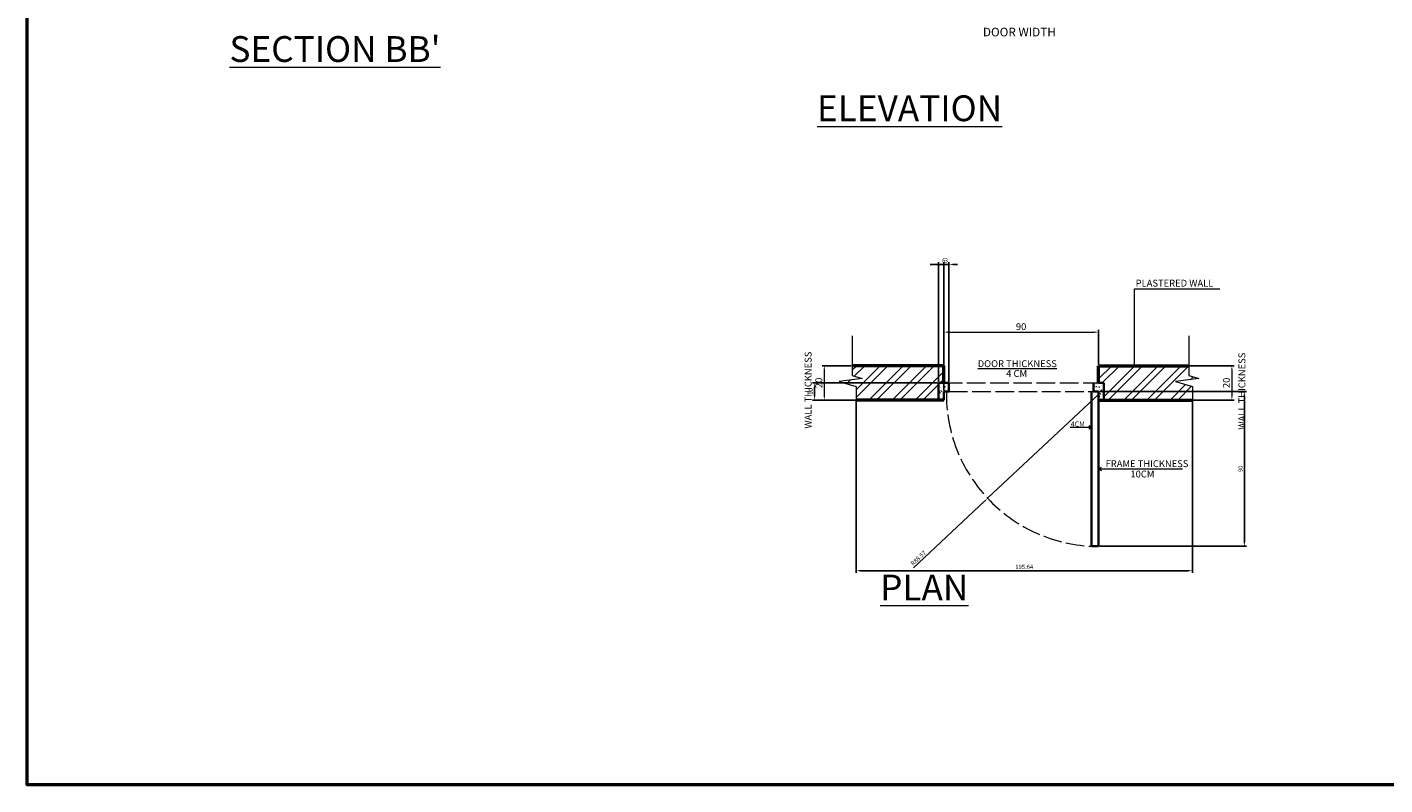
# Model space of a CAD drawing. Units: centimetres. Extents: x 1523 to 2760, y 1250 to 2134.
# Tile 1 of 4: x 1523 to 2313, y 1250 to 1691. Entities that reach past the tile are written whole.
import ezdxf

# ---------------------------------------------------------------- set-up
doc = ezdxf.new("R2010")
doc.units = ezdxf.units.CM
doc.linetypes.add('ACAD_ISO02W100', pattern=[15, 12, -3])
for name, color, linetype, lineweight in [('A-ANNO-DIMS', 2, 'Continuous', 18), ('A-ANNO-SYMB', 7, 'Continuous', 18), ('A-ANNO-TEXT', 7, 'Continuous', 18), ('A-ANNO-TTLB', 7, 'Continuous', 50), ('A-DOOR', 4, 'Continuous', 35), ('A-DOOR-OVHD', 252, 'ACAD_ISO02W100', 18), ('A-DOOR-PATT', 251, 'Continuous', 13), ('A-WALL', 7, 'Continuous', 50), ('A-WALL-PATT', 251, 'Continuous', 13)]:
    doc.layers.add(name, color=color, linetype=linetype, lineweight=lineweight)
doc.styles.get("Standard").update_dxf_attribs({"font": 'arial.ttf'})
doc.dimstyles.new('ISO-25', dxfattribs={"dimtxt": 2.5, "dimasz": 2.5, "dimexe": 1.25, "dimexo": 0.625, "dimtad": 1, "dimtxsty": 'Standard', "dimcen": 2.5, "dimadec": 0, "dimazin": 0, "dimtfac": 1, "dimtmove": 0, "dimatfit": 3, "dimfxl": 1, "dimarcsym": 0})

# ---------------------------------------------------------------- blocks, each defined once
blk = doc.blocks.new('*D1')
at = {"layer": 'A-ANNO-DIMS', "color": 0, "lineweight": -2, "transparency": 16777216}
for p, q in [((2056.32, 1494.6), (2056.32, 1514.72)), ((2146.32, 1494.6), (2146.32, 1514.72))]:
    blk.add_line(p, q, dxfattribs=at)
at = {"layer": 'A-ANNO-DIMS', "color": 0, "lineweight": 0, "transparency": 16777216}
blk.add_line((2058.82, 1513.47), (2143.82, 1513.47), dxfattribs=at)
at = {"layer": 'A-ANNO-DIMS', "color": 0, "transparency": 16777216}
for points in [[(2058.82, 1513.89), (2058.82, 1513.06), (2056.32, 1513.47)], [(2143.82, 1513.89), (2143.82, 1513.06), (2146.32, 1513.47)]]:
    blk.add_solid(points, dxfattribs=at)
at = {"layer": 'Defpoints', "color": 0, "transparency": 16777216}
for p in [(2146.32, 1513.47), (2056.32, 1493.97), (2146.32, 1493.97)]:
    blk.add_point(p, dxfattribs=at)
at = {"layer": 'A-ANNO-DIMS', "color": 0, "transparency": 16777216, "insert": (2101.32, 1516.14), "char_height": 4, "attachment_point": 5}
blk.add_mtext('90', dxfattribs=at)
blk = doc.blocks.new('*D2')
at = {"layer": 'A-ANNO-DIMS', "color": 0, "lineweight": -2, "transparency": 16777216}
for p, q in [((2199.41, 1493.97), (2225.13, 1493.97)), ((2201.6, 1473.97), (2225.13, 1473.97))]:
    blk.add_line(p, q, dxfattribs=at)
at = {"layer": 'A-ANNO-DIMS', "color": 0, "lineweight": 0, "transparency": 16777216}
blk.add_line((2223.88, 1491.47), (2223.88, 1476.47), dxfattribs=at)
at = {"layer": 'A-ANNO-DIMS', "color": 0, "transparency": 16777216}
for points in [[(2223.47, 1491.47), (2224.3, 1491.47), (2223.88, 1493.97)], [(2223.47, 1476.47), (2224.3, 1476.47), (2223.88, 1473.97)]]:
    blk.add_solid(points, dxfattribs=at)
at = {"layer": 'Defpoints', "color": 0, "transparency": 16777216}
for p in [(2198.78, 1493.97), (2200.97, 1473.97), (2223.88, 1473.97)]:
    blk.add_point(p, dxfattribs=at)
at = {"layer": 'A-ANNO-DIMS', "color": 0, "transparency": 16777216, "insert": (2221.21, 1483.97), "char_height": 4, "attachment_point": 5, "rotation": 90}
blk.add_mtext('20', dxfattribs=at)
blk = doc.blocks.new('*D3')
at = {"layer": 'A-ANNO-DIMS', "color": 0, "lineweight": -2, "transparency": 16777216}
for p, q in [((2002.51, 1493.97), (1985.59, 1493.97)), ((2004.71, 1473.97), (1985.59, 1473.97))]:
    blk.add_line(p, q, dxfattribs=at)
at = {"layer": 'A-ANNO-DIMS', "color": 0, "lineweight": 0, "transparency": 16777216}
blk.add_line((1986.84, 1491.47), (1986.84, 1476.47), dxfattribs=at)
at = {"layer": 'A-ANNO-DIMS', "color": 0, "transparency": 16777216}
for points in [[(1986.42, 1491.47), (1987.26, 1491.47), (1986.84, 1493.97)], [(1986.42, 1476.47), (1987.26, 1476.47), (1986.84, 1473.97)]]:
    blk.add_solid(points, dxfattribs=at)
at = {"layer": 'Defpoints', "color": 0, "transparency": 16777216}
for p in [(2003.14, 1493.97), (1986.84, 1473.97), (2005.33, 1473.97)]:
    blk.add_point(p, dxfattribs=at)
at = {"layer": 'A-ANNO-DIMS', "color": 0, "transparency": 16777216, "insert": (1984.17, 1483.97), "char_height": 4, "attachment_point": 5, "rotation": 90}
blk.add_mtext('20', dxfattribs=at)
blk = doc.blocks.new('BREAK-WALL-PLAN')
for p, q in [((7.67, 50.05), (7.67, 26.83)), ((13.47, 25.11), (0, 23.31)), ((7.67, 26.83), (13.47, 25.11)), ((0, 23.31), (9.86, 20.57)), ((9.86, 20.57), (9.86, 0))]:
    blk.add_line(p, q)
blk = doc.blocks.new('*D12')
at = {"layer": 'A-ANNO-DIMS', "color": 0, "lineweight": -2, "transparency": 16777216}
for p, q in [((2005.33, 1473.35), (2005.33, 1373.47)), ((2200.97, 1473.35), (2200.97, 1373.47)), ((2007.83, 1374.72), (2198.47, 1374.72))]:
    blk.add_line(p, q, dxfattribs=at)
at = {"layer": 'A-ANNO-DIMS', "color": 0, "transparency": 16777216}
for points in [[(2007.83, 1375.14), (2007.83, 1374.31), (2005.33, 1374.72)], [(2198.47, 1375.14), (2198.47, 1374.31), (2200.97, 1374.72)]]:
    blk.add_solid(points, dxfattribs=at)
at = {"layer": 'Defpoints', "color": 0, "transparency": 16777216}
for p in [(2005.33, 1473.97), (2200.97, 1473.97), (2200.97, 1374.72)]:
    blk.add_point(p, dxfattribs=at)
at = {"layer": 'A-ANNO-DIMS', "color": 0, "transparency": 16777216, "insert": (2103.15, 1376.63), "char_height": 2.5, "attachment_point": 5}
blk.add_mtext('195.64', dxfattribs=at)
blk = doc.blocks.new('*D13')
at = {"layer": 'A-ANNO-DIMS', "color": 0, "lineweight": -2, "transparency": 16777216}
for p, q in [((2146.95, 1478.97), (2232.38, 1478.97)), ((2231.13, 1476.47), (2231.13, 1391.47)), ((2146.95, 1388.97), (2232.38, 1388.97))]:
    blk.add_line(p, q, dxfattribs=at)
at = {"layer": 'A-ANNO-DIMS', "color": 0, "transparency": 16777216}
for points in [[(2230.71, 1476.47), (2231.55, 1476.47), (2231.13, 1478.97)], [(2230.71, 1391.47), (2231.55, 1391.47), (2231.13, 1388.97)]]:
    blk.add_solid(points, dxfattribs=at)
at = {"layer": 'Defpoints', "color": 0, "transparency": 16777216}
for p in [(2146.32, 1478.97), (2146.32, 1388.97), (2231.13, 1388.97)]:
    blk.add_point(p, dxfattribs=at)
at = {"layer": 'A-ANNO-DIMS', "color": 0, "transparency": 16777216, "insert": (2229.23, 1433.97), "char_height": 2.5, "attachment_point": 5, "rotation": 90}
blk.add_mtext('90', dxfattribs=at)
blk = doc.blocks.new('*D14')
at = {"layer": 'A-ANNO-DIMS', "color": 0, "lineweight": -2, "transparency": 16777216}
for p, q in [((2050.82, 1552.88), (2048.32, 1552.88)), ((2053.32, 1484.6), (2053.32, 1554.13)), ((2053.32, 1552.88), (2059.32, 1552.88)), ((2059.32, 1484.6), (2059.32, 1554.13)), ((2061.82, 1552.88), (2064.32, 1552.88))]:
    blk.add_line(p, q, dxfattribs=at)
at = {"layer": 'A-ANNO-DIMS', "color": 0, "transparency": 16777216}
for points in [[(2050.82, 1553.3), (2050.82, 1552.47), (2053.32, 1552.88)], [(2061.82, 1553.3), (2061.82, 1552.47), (2059.32, 1552.88)]]:
    blk.add_solid(points, dxfattribs=at)
at = {"layer": 'Defpoints', "color": 0, "transparency": 16777216}
for p in [(2059.32, 1552.88), (2053.32, 1483.97), (2059.32, 1483.97)]:
    blk.add_point(p, dxfattribs=at)
at = {"layer": 'A-ANNO-DIMS', "color": 0, "transparency": 16777216, "insert": (2056.32, 1554.78), "char_height": 2.5, "attachment_point": 5}
blk.add_mtext('6', dxfattribs=at)
blk = doc.blocks.new('*D15')
at = {"layer": 'A-ANNO-DIMS', "color": 0, "lineweight": -2, "transparency": 16777216}
for p, q in [((2052.7, 1483.97), (1979.97, 1483.97)), ((1981.22, 1476.47), (1981.22, 1481.47)), ((2052.7, 1473.97), (1979.97, 1473.97))]:
    blk.add_line(p, q, dxfattribs=at)
at = {"layer": 'A-ANNO-DIMS', "color": 0, "transparency": 16777216}
for points in [[(1980.8, 1481.47), (1981.63, 1481.47), (1981.22, 1483.97)], [(1980.8, 1476.47), (1981.63, 1476.47), (1981.22, 1473.97)]]:
    blk.add_solid(points, dxfattribs=at)
at = {"layer": 'Defpoints', "color": 0, "transparency": 16777216}
for p in [(1981.22, 1483.97), (2053.32, 1483.97), (2053.32, 1473.97)]:
    blk.add_point(p, dxfattribs=at)
at = {"layer": 'A-ANNO-DIMS', "color": 0, "transparency": 16777216, "insert": (1979.32, 1478.97), "char_height": 2.5, "attachment_point": 5, "rotation": 90}
blk.add_mtext('10', dxfattribs=at)
blk = doc.blocks.new('*D16')
at = {"layer": 'A-ANNO-DIMS', "color": 0, "lineweight": -2, "transparency": 16777216}
for p, q in [((2053.82, 1552.88), (2051.32, 1552.88)), ((2056.32, 1479.6), (2056.32, 1554.13)), ((2056.32, 1552.88), (2059.32, 1552.88)), ((2059.32, 1484.6), (2059.32, 1554.13)), ((2061.82, 1552.88), (2064.32, 1552.88))]:
    blk.add_line(p, q, dxfattribs=at)
at = {"layer": 'A-ANNO-DIMS', "color": 0, "transparency": 16777216}
for points in [[(2053.82, 1553.3), (2053.82, 1552.47), (2056.32, 1552.88)], [(2061.82, 1553.3), (2061.82, 1552.47), (2059.32, 1552.88)]]:
    blk.add_solid(points, dxfattribs=at)
at = {"layer": 'Defpoints', "color": 0, "transparency": 16777216}
for p in [(2059.32, 1552.88), (2056.32, 1478.97), (2059.32, 1483.97)]:
    blk.add_point(p, dxfattribs=at)
at = {"layer": 'A-ANNO-DIMS', "color": 0, "transparency": 16777216, "insert": (2057.82, 1554.78), "char_height": 2.5, "attachment_point": 5}
blk.add_mtext('3', dxfattribs=at)
blk = doc.blocks.new('*D43')
at = {"layer": 'A-ANNO-DIMS', "color": 0, "lineweight": -2, "transparency": 16777216}
for p, q in [((2146.42, 1477.45), (2081.84, 1416.83)), ((2038.69, 1376.33), (2080.01, 1415.12))]:
    blk.add_line(p, q, dxfattribs=at)
at = {"layer": 'A-ANNO-DIMS', "color": 0, "transparency": 16777216}
blk.add_solid([(2079.73, 1415.43), (2080.3, 1414.82), (2081.84, 1416.83)], dxfattribs=at)
at = {"layer": 'Defpoints', "color": 0, "transparency": 16777216}
for p in [(2146.42, 1477.45), (2081.84, 1416.83)]:
    blk.add_point(p, dxfattribs=at)
at = {"layer": 'A-ANNO-DIMS', "color": 0, "transparency": 16777216, "insert": (2041.79, 1381.85), "char_height": 2.5, "attachment_point": 5, "rotation": 43.18721}
blk.add_mtext('R88.57', dxfattribs=at)

msp = doc.modelspace()

# ---------------------------------------------------------------- hatches: boundary and pattern name
at = {"layer": 'A-DOOR-PATT'}
h = msp.add_hatch(dxfattribs=at)
h.set_pattern_fill('AR-CONC', color=256, scale=0.02)
h.paths.add_polyline_path([(2059.3227, 1483.974), (2056.3227, 1483.974), (2053.3227, 1483.974), (2053.3227, 1473.974), (2056.3227, 1473.974), (2056.3227, 1478.974), (2059.3227, 1478.974)])
h = msp.add_hatch(dxfattribs=at)
h.set_pattern_fill('AR-CONC', color=256, scale=0.02)
h.paths.add_polyline_path([(2149.3227, 1483.974), (2146.3227, 1483.974), (2143.3227, 1483.974), (2143.3227, 1478.974), (2144.8227, 1478.974), (2146.3227, 1478.974), (2146.3227, 1473.974), (2149.3227, 1473.974)])
at = {"layer": 'A-WALL-PATT'}
h = msp.add_hatch(dxfattribs=at)
h.set_pattern_fill('ANSI32', color=256)
h.paths.add_polyline_path([(2200.9735, 1481.938), (2191.1087, 1484.676), (2204.575, 1486.4753), (2198.7804, 1488.1963), (2198.7804, 1493.974), (2146.3227, 1493.974), (2146.3227, 1483.974), (2149.3227, 1483.974), (2149.3227, 1473.974), (2200.9735, 1473.974)])
h.paths.add_polyline_path([(2053.3227, 1483.974), (2056.3227, 1483.974), (2056.3227, 1493.974), (2003.1396, 1493.974), (2003.1396, 1488.1963), (2008.9342, 1486.4753), (1995.4679, 1484.676), (2005.3327, 1481.938), (2005.3327, 1473.974), (2053.3227, 1473.974)])

# ---------------------------------------------------------------- linework, layer by layer
at = {"layer": 'A-ANNO-TEXT'}
for p, q in [((2167.2635, 1493.974), (2167.2635, 1538.6326)), ((2167.2635, 1538.6326), (2216.8792, 1538.6326)), ((2142.3227, 1458.0593), (2129.873, 1458.0593)), ((2142.3227, 1458.0593), (2140.6676, 1459.0139)), ((2142.3227, 1458.0593), (2140.6676, 1457.1048)), ((2146.3227, 1433.974), (2147.9777, 1434.9286)), ((2146.3227, 1433.974), (2195.2456, 1433.974)), ((2146.3227, 1433.974), (2147.9777, 1433.0195))]:
    msp.add_line(p, q, dxfattribs=at)
at = {"layer": 'A-ANNO-TTLB'}
msp.add_lwpolyline([(1523.2447, 2133.8046), (2759.5532, 2133.8046), (2759.5532, 1250.2097), (1523.2447, 1250.2097)], close=True, dxfattribs=at)
at = {"layer": 'A-DOOR'}
for p, q in [((2056.3227, 1483.974), (2053.3227, 1483.974)), ((2053.3227, 1483.974), (2053.3227, 1473.974)), ((2056.3227, 1483.974), (2059.3227, 1483.974)), ((2056.3227, 1473.974), (2056.3227, 1478.974)), ((2056.3227, 1478.974), (2056.3227, 1473.974)), ((2056.3227, 1478.974), (2059.3917, 1478.974)), ((2059.3227, 1483.974), (2059.3227, 1478.974)), ((2142.3227, 1478.974), (2142.3227, 1388.974)), ((2143.3227, 1483.974), (2143.3227, 1478.974)), ((2146.3227, 1478.974), (2143.3227, 1478.974)), ((2146.3227, 1483.974), (2149.3227, 1483.974)), ((2146.3227, 1478.974), (2146.3227, 1473.974)), ((2146.3227, 1478.974), (2146.3227, 1388.974)), ((2149.3227, 1483.974), (2149.3227, 1473.974)), ((2142.3227, 1388.974), (2146.3227, 1388.974))]:
    msp.add_line(p, q, dxfattribs=at)
at = {"layer": 'A-DOOR-OVHD', "ltscale": 0.9}
for p, q in [((2056.3227, 1483.974), (2146.3227, 1483.974)), ((2059.3917, 1478.974), (2144.8227, 1478.974))]:
    msp.add_line(p, q, dxfattribs=at)
msp.add_arc((2146.4162, 1477.4515), 88.5721, 179.0150314, 267.3510328, dxfattribs=at)
at = {"layer": 'A-WALL'}
for p, q in [((2056.3227, 1493.974), (2003.1396, 1493.974)), ((2056.3227, 1483.974), (2056.3227, 1493.974)), ((2146.3227, 1493.974), (2198.7804, 1493.974)), ((2146.3227, 1483.974), (2146.3227, 1493.974)), ((2056.3227, 1473.974), (2005.3327, 1473.974)), ((2146.3227, 1473.974), (2200.9735, 1473.974))]:
    msp.add_line(p, q, dxfattribs=at)

# ---------------------------------------------------------------- block references
at = {"layer": 'A-ANNO-SYMB'}
for p in [(1995.468, 1461.364), (2191.1088, 1461.364)]:
    msp.add_blockref('BREAK-WALL-PLAN', p, dxfattribs=at)

# ---------------------------------------------------------------- texts
at = {"layer": 'A-ANNO-TEXT', "attachment_point": 1}
for s, width, insert, char_height in [('{\\fArial Rounded MT Bold|b0|i0|c0|p34;DOOR WIDTH}', 86.463106, (2079.089, 1690.489), 5), ("{\\fArial Rounded MT Bold|b0|i0|c0|p34;\\LSECTION BB'}", 142.942226, (1640.9164, 1685.6132), 15), ('{\\fArial Rounded MT Bold|b0|i0|c0|p34;\\LELEVATION}', 86.463106, (1982.6117, 1651.1521), 15), ('{\\fArial Rounded MT Bold|b0|i0|c0|p34;PLASTERED WALL}', 86.463106, (2167.9334, 1543.9538), 4), ('{\\fArial Rounded MT Bold|b0|i0|c0|p34;\\LDOOR THICKNESS}', 86.463106, (2076.0561, 1497.1354), 4), ('{\\fArial Rounded MT Bold|b0|i0|c0|p34;4 CM}', 86.463106, (2092.6387, 1491.4357), 4), ('{\\fArial Rounded MT Bold|b0|i0|c0|p34;4CM}', 86.463106, (2130.1711, 1461.5212), 3), ('{\\fArial Rounded MT Bold|b0|i0|c0|p34;FRAME THICKNESS}', 86.463106, (2150.4405, 1438.9729), 4), ('{\\fArial Rounded MT Bold|b0|i0|c0|p34;10CM}', 86.463106, (2164.8821, 1432.9596), 4), ('{\\fArial Rounded MT Bold|b0|i0|c0|p34;\\LPLAN}', 86.463106, (2019.3162, 1372.4557), 15)]:
    msp.add_mtext_dynamic_manual_height_columns(s, width=width, gutter_width=12.5, heights=[0], dxfattribs=dict(at, insert=insert, char_height=char_height))
at = {"layer": 'A-ANNO-TEXT', "char_height": 4, "rotation": 90}
for insert, attachment_point in [((1979.4374, 1457.3756), 7), ((2227.7118, 1456.7708), 1)]:
    msp.add_mtext_dynamic_manual_height_columns('{\\fArial Rounded MT Bold|b0|i0|c0|p34;WALL THICKNESS}', width=86.463106, gutter_width=12.5, heights=[0], dxfattribs=dict(at, insert=insert, attachment_point=attachment_point))

# ---------------------------------------------------------------- dimensions: what is measured, and where the dimension line sits
at = {"layer": 'A-ANNO-DIMS'}
for base, p1, p2, override, picture, middle in [((2059.3227, 1552.8826), (2053.3227, 1483.974), (2059.3227, 1483.974), {"dimdec": 0, "dimlfac": 1, "dimrnd": 0, "dimzin": 0, "dimdsep": 46, "dimlunit": 2}, '*D14', (2056.3227, 1554.784)), ((2059.3227, 1552.8826), (2056.3227, 1478.974), (2059.3227, 1483.974), {"dimdec": 0, "dimlfac": 1, "dimrnd": 0, "dimzin": 0, "dimdsep": 46, "dimlunit": 2}, '*D16', (2057.8227, 1554.7848)), ((2146.3227, 1513.4717), (2056.3227, 1493.974), (2146.3227, 1493.974), {"dimtxt": 4, "dimasz": 2.5, "dimclrd": 0, "dimclre": 0, "dimclrt": 0, "dimlwd": 0}, '*D1', (2101.3227, 1516.139)), ((2200.9735, 1374.724), (2005.3327, 1473.974), (2200.9735, 1473.974), {"dimdec": 2, "dimlfac": 1, "dimrnd": 0, "dimzin": 0, "dimdsep": 46, "dimlunit": 2}, '*D12', (2103.1531, 1376.6255))]:
    dim = msp.add_linear_dim(base=base, p1=p1, p2=p2, dimstyle='ISO-25', override=override, dxfattribs=at)
    dim.commit()
    dim.dimension.update_dxf_attribs({"geometry": picture, "text_midpoint": middle})
for base, p1, p2, override, picture, middle in [((1986.8394, 1473.974), (2003.1396, 1493.974), (2005.3327, 1473.974), {"dimtxt": 4, "dimclrd": 0, "dimclre": 0, "dimclrt": 0, "dimlwd": 0}, '*D3', (1984.1721, 1483.974)), ((2223.882, 1473.974), (2198.7804, 1493.974), (2200.9735, 1473.974), {"dimtxt": 4, "dimclrd": 0, "dimclre": 0, "dimclrt": 0, "dimlwd": 0}, '*D2', (2221.2147, 1483.974)), ((1981.2179, 1483.974), (2053.3227, 1473.974), (2053.3227, 1483.974), {"dimdec": 0, "dimlfac": 1, "dimrnd": 0, "dimzin": 0, "dimdsep": 46, "dimlunit": 2}, '*D15', (1979.3165, 1478.974)), ((2231.1292, 1388.974), (2146.3227, 1478.974), (2146.3227, 1388.974), {"dimdec": 0, "dimlfac": 1, "dimrnd": 0, "dimzin": 0, "dimdsep": 46, "dimlunit": 2}, '*D13', (2229.2277, 1433.974))]:
    dim = msp.add_linear_dim(base=base, p1=p1, p2=p2, angle=90, dimstyle='ISO-25', override=override, dxfattribs=at)
    dim.commit()
    dim.dimension.update_dxf_attribs({"geometry": picture, "text_midpoint": middle})
dim = msp.add_radius_dim(center=(2146.4162, 1477.4515), mpoint=(2081.8364, 1416.8341), dimstyle='ISO-25', override={"dimdec": 2, "dimlfac": 1, "dimrnd": 0, "dimzin": 0, "dimdsep": 46, "dimlunit": 2}, dxfattribs=at)
dim.commit()
dim.dimension.update_dxf_attribs({"geometry": '*D43', "text_midpoint": (2043.0885, 1380.4637), "dimtype": 164})

doc.saveas('drawing.dxf')
